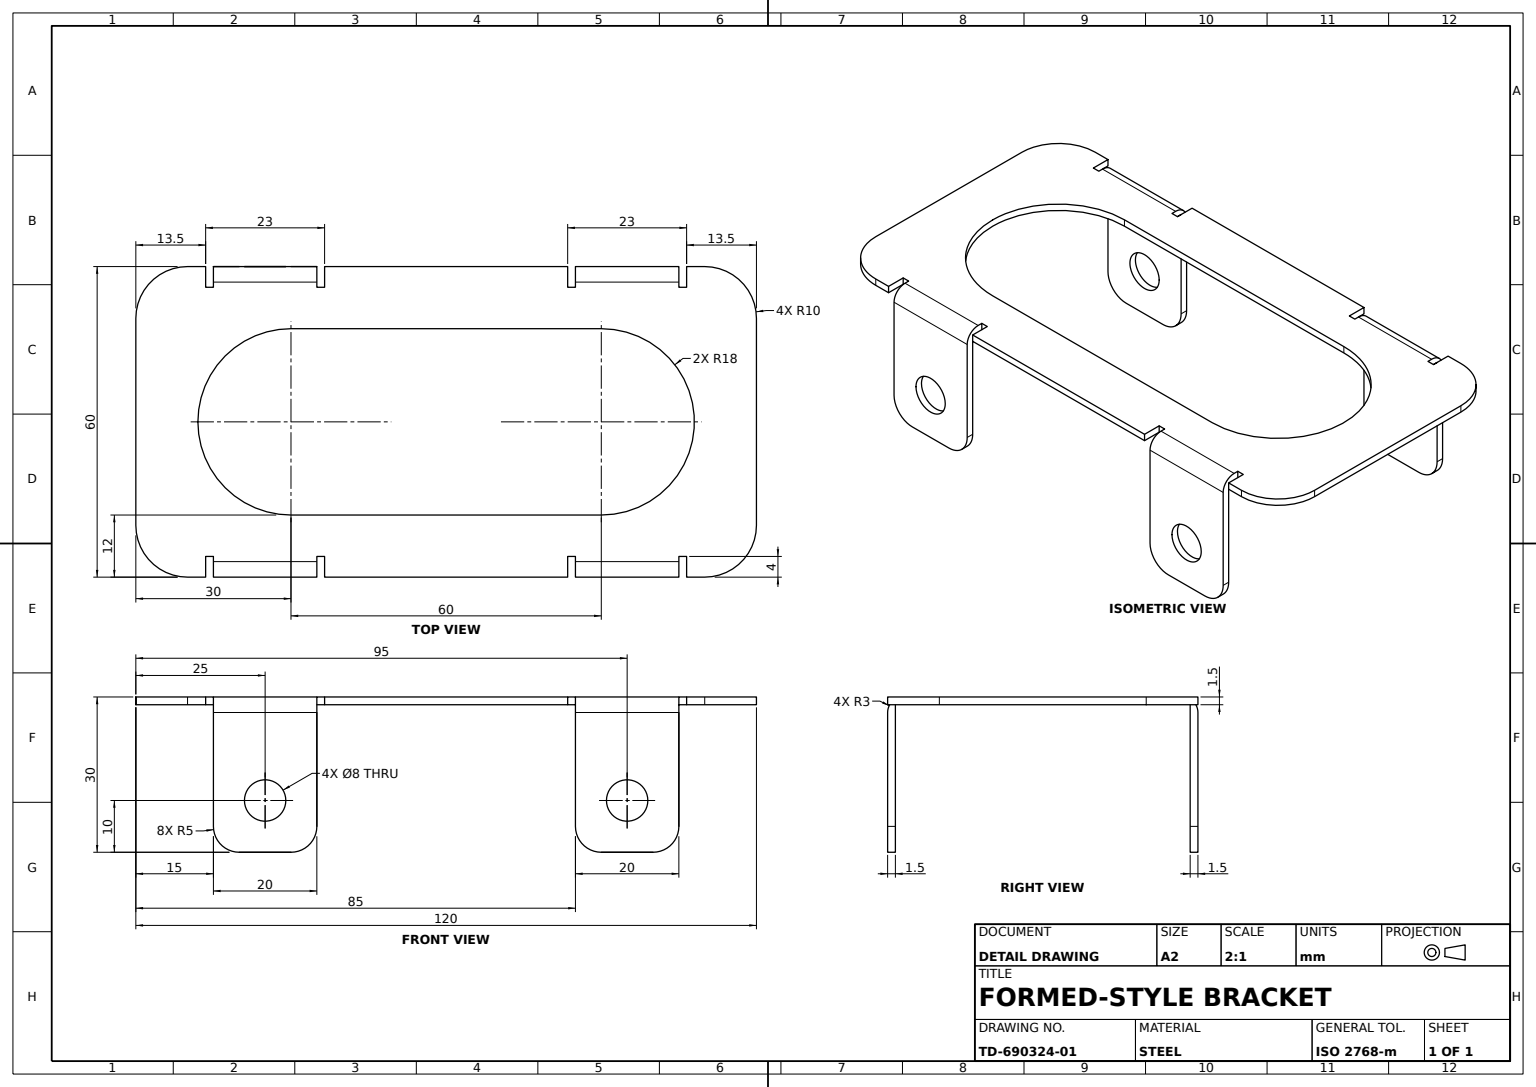
from build123d import *

# Parameters (mm, degrees)
COVER_PLATE_1_5MM_DEPTH    = 1.5
SIDE_A_LEGS_SKETCH_R       = 4
SIDE_A_MOUNTING_LEGS_DEPTH = 1.5
SIDE_START                 = -1.5
SIDE_B_LEGS_SKETCH_R       = 4
SIDE_B_MOUNTING_LEGS_DEPTH = 1.5
CORNER_FILLETS_R3_R        = 3
OBLONG_SLOT_CUT_DEPTH      = 1.5


with BuildPart() as part:
    # Cover Plate Sketch → Cover Plate 1.5mm (new body)
    with BuildSketch(Plane(origin=(0, 0, 0), x_dir=(1, 0, 0), z_dir=(0, 1, 0))):
        with BuildLine():
            Line((-30, 45), (-26, 45))
            Line((-26, 45), (-26, 46.5))
            Line((-26, 46.5), (-30, 46.5))
            Line((-30, 46.5), (-30, 50))
            ThreePointArc((-30, 50), (-27.071067812, 57.071067812), (-20, 60))
            Line((-20, 60), (20, 60))
            ThreePointArc((20, 60), (27.071067812, 57.071067812), (30, 50))
            Line((30, 50), (30, 46.5))
            Line((30, 46.5), (26, 46.5))
            Line((26, 46.5), (26, 45))
            Line((26, 45), (30, 45))
            Line((30, 45), (30, 25))
            Line((30, 25), (26, 25))
            Line((26, 25), (26, 23.5))
            Line((26, 23.5), (30, 23.5))
            Line((30, 23.5), (30, -23.5))
            Line((30, -23.5), (26, -23.5))
            Line((26, -23.5), (26, -25))
            Line((26, -25), (30, -25))
            Line((30, -25), (30, -45))
            Line((30, -45), (26, -45))
            Line((26, -45), (26, -46.5))
            Line((26, -46.5), (30, -46.5))
            Line((30, -46.5), (30, -50))
            ThreePointArc((30, -50), (27.071067812, -57.071067812), (20, -60))
            Line((20, -60), (-20, -60))
            ThreePointArc((-20, -60), (-27.071067812, -57.071067812), (-30, -50))
            Line((-30, -50), (-30, -46.5))
            Line((-30, -46.5), (-26, -46.5))
            Line((-26, -46.5), (-26, -45))
            Line((-26, -45), (-30, -45))
            Line((-30, -45), (-30, -25))
            Line((-30, -25), (-26, -25))
            Line((-26, -25), (-26, -23.5))
            Line((-26, -23.5), (-30, -23.5))
            Line((-30, -23.5), (-30, 23.5))
            Line((-30, 23.5), (-26, 23.5))
            Line((-26, 23.5), (-26, 25))
            Line((-26, 25), (-30, 25))
            Line((-30, 25), (-30, 45))
        make_face()
    extrude(amount=COVER_PLATE_1_5MM_DEPTH)

    # Side A Legs Sketch → Side A Mounting Legs (add)
    # profile 1 of 2: a face of its own
    with BuildSketch(Plane(origin=(30, 0, 0), x_dir=(0, 0, -1), z_dir=(1, 0, 0))):
        with BuildLine():
            Line((-45, 1.5), (-25, 1.5))
            Line((-25, 1.5), (-25, -23.5))
            ThreePointArc((-25, -23.5), (-26.464466094, -27.035533906), (-30, -28.5))
            Line((-30, -28.5), (-40, -28.5))
            ThreePointArc((-40, -28.5), (-43.535533906, -27.035533906), (-45, -23.5))
            Line((-45, -23.5), (-45, 1.5))
        make_face()
        with Locations((-35, -18.5)):
            Circle(SIDE_A_LEGS_SKETCH_R, mode=Mode.SUBTRACT)
    # profile 2 of 2: a face of its own
    with BuildSketch(Plane(origin=(30, 0, 0), x_dir=(0, 0, -1), z_dir=(1, 0, 0))):
        with BuildLine():
            Line((25, 1.5), (45, 1.5))
            Line((45, 1.5), (45, -23.5))
            ThreePointArc((45, -23.5), (43.535533906, -27.035533906), (40, -28.5))
            Line((40, -28.5), (30, -28.5))
            ThreePointArc((30, -28.5), (26.464466094, -27.035533906), (25, -23.5))
            Line((25, -23.5), (25, 1.5))
        make_face()
        with Locations((35, -18.5)):
            Circle(SIDE_A_LEGS_SKETCH_R, mode=Mode.SUBTRACT)
    extrude(amount=-SIDE_A_MOUNTING_LEGS_DEPTH)

    # Side B Legs Sketch → Side B Mounting Legs (add)
    # profile 1 of 2: a face of its own
    with BuildSketch(Plane.ZY.offset(30).offset(SIDE_START)):
        with BuildLine():
            Line((-45, 1.5), (-25, 1.5))
            Line((-25, 1.5), (-25, -23.5))
            ThreePointArc((-25, -23.5), (-26.464466094, -27.035533906), (-30, -28.5))
            Line((-30, -28.5), (-40, -28.5))
            ThreePointArc((-40, -28.5), (-43.535533906, -27.035533906), (-45, -23.5))
            Line((-45, -23.5), (-45, 1.5))
        make_face()
        with Locations(Location((-35, -18.5, 0), (0, 0, 180))):
            Circle(SIDE_B_LEGS_SKETCH_R, mode=Mode.SUBTRACT)
    # profile 2 of 2: a face of its own
    with BuildSketch(Plane.ZY.offset(30).offset(SIDE_START)):
        with BuildLine():
            Line((25, 1.5), (45, 1.5))
            Line((45, 1.5), (45, -23.5))
            ThreePointArc((45, -23.5), (43.535533906, -27.035533906), (40, -28.5))
            Line((40, -28.5), (30, -28.5))
            ThreePointArc((30, -28.5), (26.464466094, -27.035533906), (25, -23.5))
            Line((25, -23.5), (25, 1.5))
        make_face()
        with Locations(Location((35, -18.5, 0), (0, 0, 180))):
            Circle(SIDE_B_LEGS_SKETCH_R, mode=Mode.SUBTRACT)
    extrude(amount=SIDE_B_MOUNTING_LEGS_DEPTH)

    # Corner Fillets R3
    corner_fillets_r3_edges = [part.edges().sort_by_distance(p)[0] for p in [
        (-30, 1.5, -35),
        (-30, 1.5, 35),
        (30, 1.5, 35),
        (30, 1.5, -35),
    ]]
    fillet(corner_fillets_r3_edges, radius=CORNER_FILLETS_R3_R)

    # Oblong Slot Sketch → Oblong Slot Cut (cut)
    with BuildSketch(Plane(origin=(0, 1.5, 0), x_dir=(1, 0, 0), z_dir=(0, 1, 0))):
        with BuildLine():
            Line((-18, -30), (-18, 30))
            ThreePointArc((-18, 30), (0, 48), (18, 30))
            Line((18, 30), (18, -30))
            ThreePointArc((18, -30), (0, -48), (-18, -30))
        make_face()
    extrude(amount=-OBLONG_SLOT_CUT_DEPTH, mode=Mode.SUBTRACT)


solid = part.part
